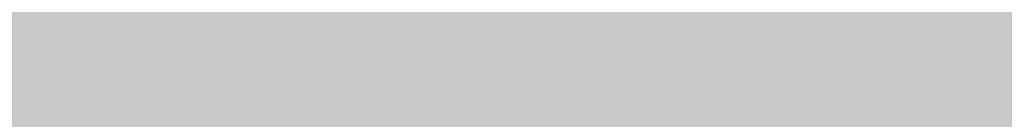
# Model space of a CAD drawing. Units: millimetres. Extents: x 0 to 2267, y 0 to 1823.
# Tile 101 of 256: x 1600.369 to 1605.705, y 1227.736 to 1228.277. Entities that reach past the tile are written whole.
import ezdxf

# ---------------------------------------------------------------- set-up
doc = ezdxf.new("R2010")
doc.units = ezdxf.units.MM
doc.header["$MEASUREMENT"] = 0
doc.layers.add('M-DIMS', color=2, linetype='Continuous', lineweight=25)
doc.layers.add('M-HATC', color=252, linetype='Continuous', lineweight=18)
doc.styles.get("Standard").update_dxf_attribs({"font": 'arial.ttf'})
doc.dimstyles.get("Standard").update_dxf_attribs({"dimtxt": 7, "dimasz": 4, "dimexe": 0.18, "dimexo": 0.0625, "dimgap": 0.09, "dimtad": 0, "dimdec": 0, "dimzin": 0, "dimdsep": 46, "dimtxsty": 'Standard', "dimcen": 0.09, "dimadec": 0, "dimazin": 0, "dimtfac": 1, "dimtdec": 0, "dimtofl": 0, "dimtmove": 0, "dimatfit": 3, "dimfxl": 1, "dimtolj": 1, "dimtzin": 0, "dimarcsym": 0})

# ---------------------------------------------------------------- blocks, each defined once
blk = doc.blocks.new('*D19')
at = {"layer": 'Defpoints', "color": 0, "transparency": 16777216}
for p in [(1605.3399, 1483.3044), (1445.5291, 1333.8851)]:
    blk.add_point(p, dxfattribs=at)
at = {"layer": 'M-DIMS', "color": 0, "lineweight": -2, "transparency": 16777216}
for p, q in [((1605.3399, 1483.2144), (1605.3399, 1483.3944)), ((1605.2499, 1483.3044), (1605.4299, 1483.3044)), ((1366.3244, 1259.8306), (1442.6072, 1331.1532))]:
    blk.add_line(p, q, dxfattribs=at)
at = {"layer": 'M-DIMS', "color": 0, "transparency": 16777216}
blk.add_solid([(1442.1519, 1331.6402), (1443.0625, 1330.6663), (1445.5291, 1333.8851)], dxfattribs=at)
at = {"layer": 'M-DIMS', "color": 0, "transparency": 16777216, "insert": (1349.6425, 1244.2335), "char_height": 7, "attachment_point": 5, "rotation": 43.0753}
blk.add_mtext('\\A1;2X R218.8', dxfattribs=at)

msp = doc.modelspace()

# ---------------------------------------------------------------- hatches: boundary and pattern name
at = {"layer": 'M-HATC'}
h = msp.add_hatch(color=256, dxfattribs=at)
h.dxf.hatch_style = 1
h.paths.add_polyline_path([(2055.771, 1603.062), (1381.0868, 1603.062), (1381.0868, 1598.062), (2055.771, 1598.062)])
h.paths.add_polyline_path([(2055.771, 1598.062), (1381.0868, 1598.062), (1381.0868, 1593.062), (2055.771, 1593.062)])
h.paths.add_polyline_path([(2051.3074, 1536.7609), (1385.5504, 1536.7609), (1385.5504, 1526.7609), (1387.5504, 1526.7609), (1388.5366, 1525.0528), (1385.3319, 1521.2335), (1385.3319, 1521.2226), (2050.2542, 1522.7491), (2048.3212, 1525.0528), (2049.3074, 1526.7609), (2051.3074, 1526.7609)])
edge = h.paths.add_edge_path()
edge.add_arc((1847.5345, 1379.1492), 135, 222.603061, 222.890851, ccw=False)
edge.add_line((1748.1663, 1287.7656), (1683.0921, 1287.7656))
edge.add_arc((1583.7239, 1379.1492), 135, 317.109149, 317.396939, ccw=False)
edge.add_arc((1678.9686, 1290.6707), 5, 222.8909, 317.1091, ccw=False)
edge.add_arc((1774.2133, 1379.1492), 135, 222.603061, 222.890851, ccw=False)
edge.add_line((1674.8451, 1287.7656), (1609.7709, 1287.7656))
edge.add_arc((1510.4027, 1379.1492), 135, 317.109149, 317.396939, ccw=False)
edge.add_arc((1605.6474, 1290.6707), 5, 222.8909, 317.1091, ccw=False)
edge.add_arc((1700.8921, 1379.1492), 135, 222.603061, 222.890851, ccw=False)
edge.add_line((1601.5239, 1287.7656), (1536.4497, 1287.7656))
edge.add_arc((1437.0815, 1379.1492), 135, 317.109149, 317.396939, ccw=False)
edge.add_arc((1532.3262, 1290.6707), 5, 222.8909, 317.1091, ccw=False)
edge.add_arc((1627.5709, 1379.1492), 135, 222.603061, 222.890851, ccw=False)
edge.add_line((1528.2027, 1287.7656), (1505.9289, 1287.7656))
edge.add_spline(control_points=[(1505.9289, 1287.7656), (1504.2622, 1287.7656), (1504.2622, 1282.7656), (1505.9289, 1282.7656)], knot_values=[0, 0, 0, 0, 5, 5, 5, 5], degree=3, periodic=0)
edge.add_line((1505.9289, 1282.7656), (1930.9289, 1282.7656))
edge.add_spline(control_points=[(1930.9289, 1282.7656), (1932.5956, 1282.7656), (1932.5956, 1287.7656), (1930.9289, 1287.7656)], knot_values=[0, 0, 0, 0, 5, 5, 5, 5], degree=3, periodic=0)
edge.add_line((1930.9289, 1287.7656), (1903.0557, 1287.7656))
edge.add_arc((1803.6875, 1379.1492), 135, 317.109149, 317.396939, ccw=False)
edge.add_arc((1898.9322, 1290.6707), 5, 222.8909, 317.1091, ccw=False)
edge.add_arc((1994.1769, 1379.1492), 135, 222.603061, 222.890851, ccw=False)
edge.add_line((1894.8087, 1287.7656), (1829.7345, 1287.7656))
edge.add_arc((1730.3663, 1379.1492), 135, 317.109149, 317.396939, ccw=False)
edge.add_arc((1825.611, 1290.6707), 5, 222.8909, 317.1091, ccw=False)
edge.add_arc((1920.8557, 1379.1492), 135, 222.603061, 222.890851, ccw=False)
edge.add_line((1821.4875, 1287.7656), (1756.4133, 1287.7656))
edge.add_arc((1657.0451, 1379.1492), 135, 317.109149, 317.396939, ccw=False)
edge.add_arc((1752.2898, 1290.6707), 5, 222.8909, 317.1091, ccw=False)
edge = h.paths.add_edge_path()
edge.add_spline(control_points=[(1843.4289, 1227.2475), (1845.0956, 1227.2475), (1845.0956, 1232.2475), (1843.4289, 1232.2475)], knot_values=[0, 0, 0, 0, 5, 5, 5, 5], degree=3, periodic=0)
edge.add_line((1843.4289, 1232.2475), (1593.4289, 1232.2475))
edge.add_spline(control_points=[(1593.4289, 1232.2475), (1591.7622, 1232.2475), (1591.7622, 1227.2475), (1593.4289, 1227.2475)], knot_values=[0, 0, 0, 0, 5, 5, 5, 5], degree=3, periodic=0)
edge.add_line((1593.4289, 1227.2475), (1843.4289, 1227.2475))
h.paths.add_polyline_path([(1905.9289, 1127.4171), (1530.9289, 1127.4171, 0.414214), (1520.9289, 1117.4171), (1530.9289, 1117.4171), (1915.9289, 1117.4171, 0.414214)])
edge = h.paths.add_edge_path()
edge.add_arc((1397.0858, 1498.4078), 12.7299, 90.78215, 190.87871, ccw=False)
edge.add_line((1396.912, 1511.1365), (1428.0097, 1511.3488))
edge.add_line((1428.0097, 1511.3488), (1433.0097, 1511.3488))
edge.add_line((1433.0097, 1511.3488), (1434.439, 1511.3488))
edge.add_arc((1419.474, 1498.0804), 20, 41.561, 74.08211)
edge.add_line((1424.9592, 1517.3135), (1399.9351, 1517.2561))
edge.add_spline(control_points=[(1399.9307, 1517.2561), (1399.884, 1517.2131), (1399.8328, 1517.1689), (1399.7774, 1517.1236)], knot_values=[11.567499, 11.567499, 11.567499, 11.567499, 11.814249, 11.814249, 11.814249, 11.814249], degree=3, periodic=0)
edge.add_spline(control_points=[(1399.6328, 1517.0099), (1399.5831, 1516.9721), (1399.5307, 1516.9338), (1399.4759, 1516.8947)], knot_values=[11.167718, 11.167718, 11.167718, 11.167718, 11.365188, 11.365188, 11.365188, 11.365188], degree=3, periodic=0)
edge.add_spline(control_points=[(1399.3398, 1516.8001), (1399.1514, 1516.6719), (1398.9384, 1516.5377), (1398.704, 1516.3994)], knot_values=[10.376405, 10.376405, 10.376405, 10.376405, 11.00994, 11.00994, 11.00994, 11.00994], degree=3, periodic=0)
edge.add_spline(control_points=[(1398.6572, 1516.3719), (1398.5789, 1516.326), (1398.4983, 1516.2797), (1398.4155, 1516.2331)], knot_values=[10.125175, 10.125175, 10.125175, 10.125175, 10.334406, 10.334406, 10.334406, 10.334406], degree=3, periodic=0)
edge.add_spline(control_points=[(1398.2642, 1516.1487), (1398.196, 1516.1111), (1398.1263, 1516.0732), (1398.0555, 1516.0351)], knot_values=[9.832246, 9.832246, 9.832246, 9.832246, 9.999658, 9.999658, 9.999658, 9.999658], degree=3, periodic=0)
edge.add_spline(control_points=[(1397.9987, 1516.0048), (1397.7312, 1515.8621), (1397.446, 1515.7171), (1397.1466, 1515.5714)], knot_values=[9.161808, 9.161808, 9.161808, 9.161808, 9.787769, 9.787769, 9.787769, 9.787769], degree=3, periodic=0)
edge.add_spline(control_points=[(1397.1466, 1515.5714), (1396.8418, 1515.423), (1396.5222, 1515.274), (1396.1914, 1515.1262)], knot_values=[8.524455, 8.524455, 8.524455, 8.524455, 9.161808, 9.161808, 9.161808, 9.161808], degree=3, periodic=0)
edge.add_spline(control_points=[(1396.0777, 1515.0756), (1395.9854, 1515.0348), (1395.8922, 1514.994), (1395.7983, 1514.9534)], knot_values=[8.275193, 8.275193, 8.275193, 8.275193, 8.451726, 8.451726, 8.451726, 8.451726], degree=3, periodic=0)
edge.add_spline(control_points=[(1395.6018, 1514.8691), (1395.4997, 1514.8257), (1395.3968, 1514.7824), (1395.2932, 1514.7394)], knot_values=[7.962917, 7.962917, 7.962917, 7.962917, 8.152764, 8.152764, 8.152764, 8.152764], degree=3, periodic=0)
edge.add_spline(control_points=[(1395.2116, 1514.7057), (1394.8278, 1514.5475), (1394.4345, 1514.3929), (1394.0364, 1514.2442)], knot_values=[7.21254, 7.21254, 7.21254, 7.21254, 7.913148, 7.913148, 7.913148, 7.913148], degree=3, periodic=0)
edge.add_spline(control_points=[(1394.0364, 1514.2442), (1393.7076, 1514.1214), (1393.3754, 1514.0027), (1393.0427, 1513.8895)], knot_values=[6.633733, 6.633733, 6.633733, 6.633733, 7.21254, 7.21254, 7.21254, 7.21254], degree=3, periodic=0)
edge.add_spline(control_points=[(1392.8214, 1513.815), (1392.7198, 1513.7812), (1392.6181, 1513.7479), (1392.5166, 1513.7152)], knot_values=[6.328796, 6.328796, 6.328796, 6.328796, 6.505493, 6.505493, 6.505493, 6.505493], degree=3, periodic=0)
edge.add_spline(control_points=[(1392.5166, 1513.7152), (1392.3187, 1513.6515), (1392.1212, 1513.59), (1391.9244, 1513.531)], knot_values=[5.984605, 5.984605, 5.984605, 5.984605, 6.328796, 6.328796, 6.328796, 6.328796], degree=3, periodic=0)
edge.add_spline(control_points=[(1391.7915, 1513.4915), (1391.3122, 1513.3501), (1390.8384, 1513.2239), (1390.3784, 1513.1171)], knot_values=[5.066697, 5.066697, 5.066697, 5.066697, 5.907055, 5.907055, 5.907055, 5.907055], degree=3, periodic=0)
edge.add_spline(control_points=[(1390.3784, 1513.1171), (1390.1797, 1513.071), (1389.9836, 1513.0284), (1389.7907, 1512.9899)], knot_values=[4.70367, 4.70367, 4.70367, 4.70367, 5.066695, 5.066695, 5.066695, 5.066695], degree=3, periodic=0)
edge.add_spline(control_points=[(1389.422, 1512.9204), (1389.2459, 1512.8892), (1389.0729, 1512.8617), (1388.9036, 1512.8381)], knot_values=[4.130571, 4.130571, 4.130571, 4.130571, 4.469816, 4.469816, 4.469816, 4.469816], degree=3, periodic=0)
edge.add_spline(control_points=[(1388.9036, 1512.8381), (1388.591, 1512.7946), (1388.2911, 1512.7644), (1388.0071, 1512.7494)], knot_values=[3.504031, 3.504031, 3.504031, 3.504031, 4.130571, 4.130571, 4.130571, 4.130571], degree=3, periodic=0)
edge.add_spline(control_points=[(1387.9356, 1512.7459), (1387.8538, 1512.7423), (1387.7733, 1512.74), (1387.6944, 1512.739)], knot_values=[3.268866, 3.268866, 3.268866, 3.268866, 3.451164, 3.451164, 3.451164, 3.451164], degree=3, periodic=0)
edge.add_spline(control_points=[(1387.3351, 1512.7443), (1387.2076, 1512.7499), (1387.0847, 1512.7597), (1386.967, 1512.7739)], knot_values=[2.670686, 2.670686, 2.670686, 2.670686, 2.984, 2.984, 2.984, 2.984], degree=3, periodic=0)
edge.add_spline(control_points=[(1386.8327, 1512.7922), (1386.8209, 1512.7941), (1386.8092, 1512.7959), (1386.7975, 1512.7979)], knot_values=[2.516981, 2.516981, 2.516981, 2.516981, 2.549528, 2.549528, 2.549528, 2.549528], degree=3, periodic=0)
edge.add_spline(control_points=[(1386.4526, 1512.8735), (1386.4257, 1512.881), (1386.3993, 1512.889), (1386.3733, 1512.8972)], knot_values=[2.095869, 2.095869, 2.095869, 2.095869, 2.17941, 2.17941, 2.17941, 2.17941], degree=3, periodic=0)
edge.add_spline(control_points=[(1386.0691, 1513.0189), (1386.0634, 1513.0217), (1386.0577, 1513.0246), (1386.052, 1513.0275)], knot_values=[1.72453, 1.72453, 1.72453, 1.72453, 1.745933, 1.745933, 1.745933, 1.745933], degree=3, periodic=0)
edge.add_arc((1399.474, 1498.0804), 20, 131.82432, 180)
edge.add_arc((1630.3336, 1505.5484), 250.9708, 181.705176, 236.427975)
edge.add_arc((1605.3399, 1483.3044), 218.7822, 238.660829, 243.34961)
edge.add_arc((1647.0911, 1510.3592), 262.8986, 183.129836, 237.853442, ccw=False)
h.paths.add_polyline_path([(1406.5369, 1391.9644, 0.149382), (1491.5506, 1296.4418, -0.129517)], flags=17)
edge = h.paths.add_edge_path()
edge.add_arc((2037.3838, 1498.0804), 20, 0, 48.26587)
edge.add_spline(control_points=[(2050.6973, 1513.0052), (2050.6512, 1512.9847), (2050.6034, 1512.9655), (2050.5539, 1512.9477)], knot_values=[1.835652, 1.835652, 1.835652, 1.835652, 2.000781, 2.000781, 2.000781, 2.000781], degree=3, periodic=0)
edge.add_spline(control_points=[(2050.4616, 1512.9166), (2050.479, 1512.9221), (2050.4963, 1512.9277), (2050.5133, 1512.9335)], knot_values=[2.045477, 2.045477, 2.045477, 2.045477, 2.101389, 2.101389, 2.101389, 2.101389], degree=3, periodic=0)
edge.add_spline(control_points=[(2050.129, 1512.8342), (2050.1984, 1512.8473), (2050.2657, 1512.8623), (2050.3308, 1512.8792)], knot_values=[2.237629, 2.237629, 2.237629, 2.237629, 2.435841, 2.435841, 2.435841, 2.435841], degree=3, periodic=0)
edge.add_spline(control_points=[(2050.0946, 1512.8278), (2050.1061, 1512.8299), (2050.1176, 1512.832), (2050.129, 1512.8342)], knot_values=[2.435841, 2.435841, 2.435841, 2.435841, 2.468321, 2.468321, 2.468321, 2.468321], degree=3, periodic=0)
edge.add_spline(control_points=[(2049.7843, 1512.7851), (2049.8552, 1512.7922), (2049.9243, 1512.8008), (2049.9917, 1512.8109)], knot_values=[2.563852, 2.563852, 2.563852, 2.563852, 2.748541, 2.748541, 2.748541, 2.748541], degree=3, periodic=0)
edge.add_spline(control_points=[(2049.4052, 1512.7617), (2049.5364, 1512.7653), (2049.6629, 1512.773), (2049.7843, 1512.7851)], knot_values=[2.748541, 2.748541, 2.748541, 2.748541, 3.064882, 3.064882, 3.064882, 3.064882], degree=3, periodic=0)
edge.add_spline(control_points=[(2049.1698, 1512.7597), (2049.2336, 1512.7591), (2049.2965, 1512.7594), (2049.3584, 1512.7606)], knot_values=[3.102309, 3.102309, 3.102309, 3.102309, 3.2503, 3.2503, 3.2503, 3.2503], degree=3, periodic=0)
edge.add_spline(control_points=[(2048.8573, 1512.7691), (2048.9638, 1512.7638), (2049.068, 1512.7606), (2049.1698, 1512.7597)], knot_values=[3.2503, 3.2503, 3.2503, 3.2503, 3.486069, 3.486069, 3.486069, 3.486069], degree=3, periodic=0)
edge.add_spline(control_points=[(2048.6924, 1512.7789), (2048.3729, 1512.8009), (2048.0345, 1512.8411), (2047.6817, 1512.897)], knot_values=[3.606429, 3.606429, 3.606429, 3.606429, 4.2989, 4.2989, 4.2989, 4.2989], degree=3, periodic=0)
edge.add_spline(control_points=[(2047.6817, 1512.897), (2047.5458, 1512.9185), (2047.4077, 1512.9424), (2047.2678, 1512.9685)], knot_values=[4.2989, 4.2989, 4.2989, 4.2989, 4.565769, 4.565769, 4.565769, 4.565769], degree=3, periodic=0)
edge.add_spline(control_points=[(2047.2678, 1512.9685), (2047.1449, 1512.9914), (2047.0207, 1513.016), (2046.8951, 1513.0422)], knot_values=[4.565769, 4.565769, 4.565769, 4.565769, 4.799971, 4.799971, 4.799971, 4.799971], degree=3, periodic=0)
edge.add_spline(control_points=[(2046.8951, 1513.0422), (2046.5286, 1513.1188), (2046.1513, 1513.209), (2045.7676, 1513.3107)], knot_values=[4.799971, 4.799971, 4.799971, 4.799971, 5.483718, 5.483718, 5.483718, 5.483718], degree=3, periodic=0)
edge.add_spline(control_points=[(2045.7676, 1513.3107), (2045.3724, 1513.4154), (2044.9704, 1513.5322), (2044.5662, 1513.6588)], knot_values=[5.483718, 5.483718, 5.483718, 5.483718, 6.187866, 6.187866, 6.187866, 6.187866], degree=3, periodic=0)
edge.add_spline(control_points=[(2044.5662, 1513.6588), (2044.4149, 1513.7061), (2044.2633, 1513.7549), (2044.1116, 1513.8048)], knot_values=[6.187866, 6.187866, 6.187866, 6.187866, 6.451551, 6.451551, 6.451551, 6.451551], degree=3, periodic=0)
edge.add_spline(control_points=[(2044.1116, 1513.8048), (2043.9967, 1513.8427), (2043.8817, 1513.8813), (2043.7668, 1513.9205)], knot_values=[6.451551, 6.451551, 6.451551, 6.451551, 6.651434, 6.651434, 6.651434, 6.651434], degree=3, periodic=0)
edge.add_spline(control_points=[(2043.7668, 1513.9205), (2043.3716, 1514.0554), (2042.9774, 1514.1979), (2042.5886, 1514.3458)], knot_values=[6.651434, 6.651434, 6.651434, 6.651434, 7.338879, 7.338879, 7.338879, 7.338879], degree=3, periodic=0)
edge.add_spline(control_points=[(2042.5886, 1514.3458), (2042.1643, 1514.5071), (2041.7465, 1514.6749), (2041.3409, 1514.846)], knot_values=[7.338879, 7.338879, 7.338879, 7.338879, 8.089209, 8.089209, 8.089209, 8.089209], degree=3, periodic=0)
edge.add_spline(control_points=[(2041.3409, 1514.846), (2041.1028, 1514.9465), (2040.869, 1515.0481), (2040.6405, 1515.1502)], knot_values=[8.089209, 8.089209, 8.089209, 8.089209, 8.529587, 8.529587, 8.529587, 8.529587], degree=3, periodic=0)
edge.add_spline(control_points=[(2040.51, 1515.2089), (2040.0824, 1515.4022), (2039.6747, 1515.5971), (2039.295, 1515.7894)], knot_values=[8.613818, 8.613818, 8.613818, 8.613818, 9.44571, 9.44571, 9.44571, 9.44571], degree=3, periodic=0)
edge.add_spline(control_points=[(2039.295, 1515.7894), (2039.0618, 1515.9075), (2038.8391, 1516.0246), (2038.6288, 1516.1398)], knot_values=[9.44571, 9.44571, 9.44571, 9.44571, 9.956404, 9.956404, 9.956404, 9.956404], degree=3, periodic=0)
edge.add_spline(control_points=[(2038.6288, 1516.1398), (2038.5187, 1516.2001), (2038.4121, 1516.2598), (2038.309, 1516.3189)], knot_values=[9.956404, 9.956404, 9.956404, 9.956404, 10.223542, 10.223542, 10.223542, 10.223542], degree=3, periodic=0)
edge.add_spline(control_points=[(2038.309, 1516.3189), (2038.2138, 1516.3735), (2038.1216, 1516.4276), (2038.0328, 1516.481)], knot_values=[10.223542, 10.223542, 10.223542, 10.223542, 10.47051, 10.47051, 10.47051, 10.47051], degree=3, periodic=0)
edge.add_spline(control_points=[(2038.0328, 1516.481), (2037.7855, 1516.6296), (2037.5639, 1516.773), (2037.3722, 1516.909)], knot_values=[10.47051, 10.47051, 10.47051, 10.47051, 11.15767, 11.15767, 11.15767, 11.15767], degree=3, periodic=0)
edge.add_spline(control_points=[(2037.3722, 1516.909), (2037.2789, 1516.9752), (2037.1927, 1517.0396), (2037.1142, 1517.102)], knot_values=[11.15767, 11.15767, 11.15767, 11.15767, 11.49227, 11.49227, 11.49227, 11.49227], degree=3, periodic=0)
edge.add_spline(control_points=[(2036.8564, 1517.3259), (2036.9148, 1517.2692), (2036.9814, 1517.2103), (2037.0557, 1517.1492)], knot_values=[11.577341, 11.577341, 11.577341, 11.577341, 11.91035, 11.91035, 11.91035, 11.91035], degree=3, periodic=0)
edge.add_spline(control_points=[(2036.8074, 1517.3748), (2036.823, 1517.3587), (2036.8393, 1517.3424), (2036.8564, 1517.3259)], knot_values=[11.91035, 11.91035, 11.91035, 11.91035, 12.007402, 12.007402, 12.007402, 12.007402], degree=3, periodic=0)
edge.add_spline(control_points=[(2036.7017, 1517.494), (2036.7104, 1517.483), (2036.7196, 1517.4719), (2036.7291, 1517.4606)], knot_values=[12.184155, 12.184155, 12.184155, 12.184155, 12.255409, 12.255409, 12.255409, 12.255409], degree=3, periodic=0)
edge.add_spline(control_points=[(2036.6159, 1517.6205), (2036.62, 1517.613), (2036.6243, 1517.6055), (2036.6289, 1517.5979)], knot_values=[12.487913, 12.487913, 12.487913, 12.487913, 12.541035, 12.541035, 12.541035, 12.541035], degree=3, periodic=0)
edge.add_spline(control_points=[(2036.5635, 1517.786), (2036.5637, 1517.7794), (2036.5642, 1517.7726), (2036.565, 1517.7658)], knot_values=[12.911761, 12.911761, 12.911761, 12.911761, 12.968286, 12.968286, 12.968286, 12.968286], degree=3, periodic=0)
edge.add_spline(control_points=[(2036.6166, 1517.9304), (2036.6125, 1517.9259), (2036.6086, 1517.9212), (2036.6049, 1517.9165)], knot_values=[13.382527, 13.382527, 13.382527, 13.382527, 13.433791, 13.433791, 13.433791, 13.433791], degree=3, periodic=0)
edge.add_spline(control_points=[(2036.749, 1518.017), (2036.7361, 1518.0116), (2036.7239, 1518.006), (2036.7124, 1518.0002)], knot_values=[13.726299, 13.726299, 13.726299, 13.726299, 13.809928, 13.809928, 13.809928, 13.809928], degree=3, periodic=0)
edge.add_spline(control_points=[(2036.8604, 1518.0528), (2036.8386, 1518.0474), (2036.8181, 1518.0416), (2036.7988, 1518.0353)], knot_values=[13.910887, 13.910887, 13.910887, 13.910887, 14.02153, 14.02153, 14.02153, 14.02153], degree=3, periodic=0)
edge.add_line((2036.9639, 1518.0804), (2032.3838, 1518.0804))
edge.add_line((2032.3838, 1518.0804), (2027.3838, 1518.0804))
edge.add_line((2027.3838, 1518.0804), (2022.3838, 1518.0804))
edge.add_line((2022.3838, 1518.0804), (2017.3838, 1518.0804))
edge.add_arc((2017.3838, 1498.0804), 20, 90, 138.439)
edge.add_line((2002.4188, 1511.3488), (2003.8481, 1511.3488))
edge.add_line((2003.8481, 1511.3488), (2008.8481, 1511.3488))
edge.add_line((2008.8481, 1511.3488), (2039.772, 1511.1377))
edge.add_arc((2039.772, 1498.4078), 12.7299, -10.87871, 90, ccw=False)
edge.add_arc((1789.7668, 1510.3592), 262.8986, 302.146558, 356.870164, ccw=False)
edge.add_arc((1831.5179, 1483.3044), 218.7822, 296.65039, 301.339171)
edge.add_arc((1806.5242, 1505.5484), 250.9708, 303.572025, 358.294824)
h.paths.add_polyline_path([(2030.321, 1391.9644, -0.129517), (1945.3072, 1296.4418, 0.149382)], flags=17)
edge = h.paths.add_edge_path()
edge.add_spline(control_points=[(2037.2464, 1518.0821), (2037.2898, 1518.081), (2037.3355, 1518.0804), (2037.3838, 1518.0804)], knot_values=[0.000012, 0.000012, 0.000012, 0.000012, 0.144754, 0.144754, 0.144754, 0.144754], degree=3, periodic=0)
edge.add_line((2037.3357, 1518.0804), (2037.0096, 1518.0804))
edge.add_spline(control_points=[(2037.0096, 1518.0804), (2036.9822, 1518.0768), (2036.956, 1518.0727), (2036.9312, 1518.0681)], knot_values=[14.13465, 14.13465, 14.13465, 14.13465, 14.247197, 14.247197, 14.247197, 14.247197], degree=3, periodic=0)
edge.add_spline(control_points=[(2036.9312, 1518.0681), (2036.9276, 1518.0674), (2036.9241, 1518.0667), (2036.9205, 1518.0661)], knot_values=[14.118315, 14.118315, 14.118315, 14.118315, 14.13465, 14.13465, 14.13465, 14.13465], degree=3, periodic=0)
edge.add_spline(control_points=[(2036.9205, 1518.0661), (2036.9118, 1518.0644), (2036.9032, 1518.0626), (2036.8948, 1518.0608)], knot_values=[14.078086, 14.078086, 14.078086, 14.078086, 14.118315, 14.118315, 14.118315, 14.118315], degree=3, periodic=0)
edge.add_spline(control_points=[(2036.8948, 1518.0608), (2036.883, 1518.0583), (2036.8716, 1518.0556), (2036.8604, 1518.0528)], knot_values=[14.02153, 14.02153, 14.02153, 14.02153, 14.078086, 14.078086, 14.078086, 14.078086], degree=3, periodic=0)
edge.add_spline(control_points=[(2036.8604, 1518.0528), (2036.8386, 1518.0474), (2036.8181, 1518.0416), (2036.7988, 1518.0353)], knot_values=[13.910887, 13.910887, 13.910887, 13.910887, 14.02153, 14.02153, 14.02153, 14.02153], degree=3, periodic=0)
edge.add_spline(control_points=[(2036.7988, 1518.0353), (2036.7981, 1518.035), (2036.7974, 1518.0348), (2036.7967, 1518.0346)], knot_values=[13.906906, 13.906906, 13.906906, 13.906906, 13.910887, 13.910887, 13.910887, 13.910887], degree=3, periodic=0)
edge.add_spline(control_points=[(2036.7967, 1518.0346), (2036.7882, 1518.0318), (2036.7799, 1518.0289), (2036.7719, 1518.0259)], knot_values=[13.857826, 13.857826, 13.857826, 13.857826, 13.906906, 13.906906, 13.906906, 13.906906], degree=3, periodic=0)
edge.add_spline(control_points=[(2036.7719, 1518.0259), (2036.764, 1518.023), (2036.7564, 1518.02), (2036.749, 1518.017)], knot_values=[13.809928, 13.809928, 13.809928, 13.809928, 13.857826, 13.857826, 13.857826, 13.857826], degree=3, periodic=0)
edge.add_spline(control_points=[(2036.749, 1518.017), (2036.7361, 1518.0116), (2036.7239, 1518.006), (2036.7124, 1518.0002)], knot_values=[13.726299, 13.726299, 13.726299, 13.726299, 13.809928, 13.809928, 13.809928, 13.809928], degree=3, periodic=0)
edge.add_spline(control_points=[(2036.7124, 1518.0002), (2036.7121, 1518), (2036.7118, 1517.9999), (2036.7115, 1517.9997)], knot_values=[13.723993, 13.723993, 13.723993, 13.723993, 13.726299, 13.726299, 13.726299, 13.726299], degree=3, periodic=0)
edge.add_spline(control_points=[(2036.7115, 1517.9997), (2036.7063, 1517.9971), (2036.7013, 1517.9944), (2036.6965, 1517.9917)], knot_values=[13.686536, 13.686536, 13.686536, 13.686536, 13.723993, 13.723993, 13.723993, 13.723993], degree=3, periodic=0)
edge.add_spline(control_points=[(2036.6965, 1517.9917), (2036.6919, 1517.9891), (2036.6874, 1517.9865), (2036.6831, 1517.9839)], knot_values=[13.651251, 13.651251, 13.651251, 13.651251, 13.686536, 13.686536, 13.686536, 13.686536], degree=3, periodic=0)
edge.add_spline(control_points=[(2036.6831, 1517.9839), (2036.6764, 1517.9798), (2036.67, 1517.9757), (2036.6639, 1517.9714)], knot_values=[13.596804, 13.596804, 13.596804, 13.596804, 13.651251, 13.651251, 13.651251, 13.651251], degree=3, periodic=0)
edge.add_spline(control_points=[(2036.6639, 1517.9714), (2036.6636, 1517.9712), (2036.6633, 1517.9709), (2036.6629, 1517.9707)], knot_values=[13.593956, 13.593956, 13.593956, 13.593956, 13.596804, 13.596804, 13.596804, 13.596804], degree=3, periodic=0)
edge.add_spline(control_points=[(2036.6629, 1517.9707), (2036.6603, 1517.9689), (2036.6577, 1517.967), (2036.6552, 1517.9651)], knot_values=[13.570322, 13.570322, 13.570322, 13.570322, 13.593956, 13.593956, 13.593956, 13.593956], degree=3, periodic=0)
edge.add_spline(control_points=[(2036.6552, 1517.9651), (2036.6525, 1517.9631), (2036.6499, 1517.9611), (2036.6474, 1517.9591)], knot_values=[13.545477, 13.545477, 13.545477, 13.545477, 13.570322, 13.570322, 13.570322, 13.570322], degree=3, periodic=0)
edge.add_spline(control_points=[(2036.6474, 1517.9591), (2036.6472, 1517.9589), (2036.6471, 1517.9588), (2036.6469, 1517.9587)], knot_values=[13.543931, 13.543931, 13.543931, 13.543931, 13.545477, 13.545477, 13.545477, 13.545477], degree=3, periodic=0)
edge.add_spline(control_points=[(2036.6469, 1517.9587), (2036.6412, 1517.9541), (2036.6358, 1517.9494), (2036.6307, 1517.9447)], knot_values=[13.488237, 13.488237, 13.488237, 13.488237, 13.543931, 13.543931, 13.543931, 13.543931], degree=3, periodic=0)
edge.add_spline(control_points=[(2036.6307, 1517.9447), (2036.6282, 1517.9423), (2036.6257, 1517.9399), (2036.6233, 1517.9374)], knot_values=[13.460307, 13.460307, 13.460307, 13.460307, 13.488237, 13.488237, 13.488237, 13.488237], degree=3, periodic=0)
edge.add_spline(control_points=[(2036.6233, 1517.9374), (2036.6215, 1517.9356), (2036.6198, 1517.9338), (2036.6181, 1517.932)], knot_values=[13.439712, 13.439712, 13.439712, 13.439712, 13.460307, 13.460307, 13.460307, 13.460307], degree=3, periodic=0)
edge.add_spline(control_points=[(2036.6181, 1517.932), (2036.6176, 1517.9315), (2036.6171, 1517.9309), (2036.6166, 1517.9304)], knot_values=[13.433791, 13.433791, 13.433791, 13.433791, 13.439712, 13.439712, 13.439712, 13.439712], degree=3, periodic=0)
edge.add_spline(control_points=[(2036.6166, 1517.9304), (2036.6125, 1517.9259), (2036.6086, 1517.9212), (2036.6049, 1517.9165)], knot_values=[13.382527, 13.382527, 13.382527, 13.382527, 13.433791, 13.433791, 13.433791, 13.433791], degree=3, periodic=0)
edge.add_spline(control_points=[(2036.6049, 1517.9165), (2036.6026, 1517.9135), (2036.6004, 1517.9104), (2036.5982, 1517.9074)], knot_values=[13.350017, 13.350017, 13.350017, 13.350017, 13.382527, 13.382527, 13.382527, 13.382527], degree=3, periodic=0)
edge.add_spline(control_points=[(2036.5982, 1517.9074), (2036.5972, 1517.9059), (2036.5962, 1517.9043), (2036.5952, 1517.9028)], knot_values=[13.333922, 13.333922, 13.333922, 13.333922, 13.350017, 13.350017, 13.350017, 13.350017], degree=3, periodic=0)
edge.add_spline(control_points=[(2036.5952, 1517.9028), (2036.5945, 1517.9018), (2036.5939, 1517.9009), (2036.5933, 1517.8999)], knot_values=[13.323828, 13.323828, 13.323828, 13.323828, 13.333922, 13.333922, 13.333922, 13.333922], degree=3, periodic=0)
edge.add_spline(control_points=[(2036.5933, 1517.8999), (2036.5905, 1517.8955), (2036.5879, 1517.8909), (2036.5855, 1517.8864)], knot_values=[13.277545, 13.277545, 13.277545, 13.277545, 13.323828, 13.323828, 13.323828, 13.323828], degree=3, periodic=0)
edge.add_spline(control_points=[(2036.5855, 1517.8864), (2036.5836, 1517.8827), (2036.5817, 1517.8789), (2036.5801, 1517.8751)], knot_values=[13.240119, 13.240119, 13.240119, 13.240119, 13.277545, 13.277545, 13.277545, 13.277545], degree=3, periodic=0)
edge.add_spline(control_points=[(2036.5801, 1517.8751), (2036.5795, 1517.8739), (2036.579, 1517.8727), (2036.5785, 1517.8715)], knot_values=[13.228211, 13.228211, 13.228211, 13.228211, 13.240119, 13.240119, 13.240119, 13.240119], degree=3, periodic=0)
edge.add_spline(control_points=[(2036.5785, 1517.8715), (2036.578, 1517.8702), (2036.5774, 1517.869), (2036.5769, 1517.8677)], knot_values=[13.215717, 13.215717, 13.215717, 13.215717, 13.228211, 13.228211, 13.228211, 13.228211], degree=3, periodic=0)
edge.add_spline(control_points=[(2036.5769, 1517.8677), (2036.5755, 1517.864), (2036.5741, 1517.8603), (2036.5729, 1517.8565)], knot_values=[13.179847, 13.179847, 13.179847, 13.179847, 13.215717, 13.215717, 13.215717, 13.215717], degree=3, periodic=0)
edge.add_spline(control_points=[(2036.5729, 1517.8565), (2036.5713, 1517.8515), (2036.5699, 1517.8464), (2036.5687, 1517.8413)], knot_values=[13.132017, 13.132017, 13.132017, 13.132017, 13.179847, 13.179847, 13.179847, 13.179847], degree=3, periodic=0)
edge.add_spline(control_points=[(2036.5687, 1517.8413), (2036.5684, 1517.8402), (2036.5682, 1517.8392), (2036.568, 1517.8382)], knot_values=[13.122482, 13.122482, 13.122482, 13.122482, 13.132017, 13.132017, 13.132017, 13.132017], degree=3, periodic=0)
edge.add_spline(control_points=[(2036.568, 1517.8382), (2036.5676, 1517.8363), (2036.5672, 1517.8345), (2036.5669, 1517.8327)], knot_values=[13.105592, 13.105592, 13.105592, 13.105592, 13.122482, 13.122482, 13.122482, 13.122482], degree=3, periodic=0)
edge.add_spline(control_points=[(2036.5669, 1517.8327), (2036.5662, 1517.8292), (2036.5657, 1517.8257), (2036.5652, 1517.8222)], knot_values=[13.074063, 13.074063, 13.074063, 13.074063, 13.105592, 13.105592, 13.105592, 13.105592], degree=3, periodic=0)
edge.add_spline(control_points=[(2036.5652, 1517.8222), (2036.5652, 1517.8222), (2036.5652, 1517.8222), (2036.5652, 1517.8222)], knot_values=[13.074043, 13.074043, 13.074043, 13.074043, 13.074063, 13.074063, 13.074063, 13.074063], degree=3, periodic=0)
edge.add_spline(control_points=[(2036.5652, 1517.8222), (2036.5644, 1517.8164), (2036.5639, 1517.8106), (2036.5636, 1517.8046)], knot_values=[13.021884, 13.021884, 13.021884, 13.021884, 13.074043, 13.074043, 13.074043, 13.074043], degree=3, periodic=0)
edge.add_spline(control_points=[(2036.5636, 1517.8046), (2036.5636, 1517.804), (2036.5636, 1517.8034), (2036.5635, 1517.8028)], knot_values=[13.01674, 13.01674, 13.01674, 13.01674, 13.021884, 13.021884, 13.021884, 13.021884], degree=3, periodic=0)
edge.add_spline(control_points=[(2036.5635, 1517.8028), (2036.5634, 1517.8005), (2036.5634, 1517.7982), (2036.5634, 1517.7958)], knot_values=[12.996438, 12.996438, 12.996438, 12.996438, 13.01674, 13.01674, 13.01674, 13.01674], degree=3, periodic=0)
edge.add_spline(control_points=[(2036.5634, 1517.7958), (2036.5633, 1517.7926), (2036.5634, 1517.7893), (2036.5635, 1517.786)], knot_values=[12.968286, 12.968286, 12.968286, 12.968286, 12.996438, 12.996438, 12.996438, 12.996438], degree=3, periodic=0)
edge.add_spline(control_points=[(2036.5635, 1517.786), (2036.5637, 1517.7794), (2036.5642, 1517.7726), (2036.565, 1517.7658)], knot_values=[12.911761, 12.911761, 12.911761, 12.911761, 12.968286, 12.968286, 12.968286, 12.968286], degree=3, periodic=0)
edge.add_spline(control_points=[(2036.565, 1517.7658), (2036.565, 1517.7657), (2036.565, 1517.7656), (2036.565, 1517.7656)], knot_values=[12.911017, 12.911017, 12.911017, 12.911017, 12.911761, 12.911761, 12.911761, 12.911761], degree=3, periodic=0)
edge.add_spline(control_points=[(2036.565, 1517.7656), (2036.5654, 1517.7625), (2036.5658, 1517.7593), (2036.5663, 1517.7562)], knot_values=[12.88528, 12.88528, 12.88528, 12.88528, 12.911017, 12.911017, 12.911017, 12.911017], degree=3, periodic=0)
edge.add_spline(control_points=[(2036.5663, 1517.7562), (2036.5667, 1517.7534), (2036.5672, 1517.7506), (2036.5677, 1517.7478)], knot_values=[12.862519, 12.862519, 12.862519, 12.862519, 12.88528, 12.88528, 12.88528, 12.88528], degree=3, periodic=0)
edge.add_spline(control_points=[(2036.5677, 1517.7478), (2036.5678, 1517.7474), (2036.5679, 1517.7469), (2036.568, 1517.7465)], knot_values=[12.858885, 12.858885, 12.858885, 12.858885, 12.862519, 12.862519, 12.862519, 12.862519], degree=3, periodic=0)
edge.add_spline(control_points=[(2036.568, 1517.7465), (2036.5692, 1517.7399), (2036.5707, 1517.7332), (2036.5724, 1517.7264)], knot_values=[12.8053, 12.8053, 12.8053, 12.8053, 12.858885, 12.858885, 12.858885, 12.858885], degree=3, periodic=0)
edge.add_spline(control_points=[(2036.5724, 1517.7264), (2036.5734, 1517.7226), (2036.5745, 1517.7187), (2036.5756, 1517.7149)], knot_values=[12.775176, 12.775176, 12.775176, 12.775176, 12.8053, 12.8053, 12.8053, 12.8053], degree=3, periodic=0)
edge.add_spline(control_points=[(2036.5756, 1517.7149), (2036.5763, 1517.7125), (2036.577, 1517.7102), (2036.5778, 1517.7078)], knot_values=[12.756759, 12.756759, 12.756759, 12.756759, 12.775176, 12.775176, 12.775176, 12.775176], degree=3, periodic=0)
edge.add_spline(control_points=[(2036.5778, 1517.7078), (2036.5781, 1517.7067), (2036.5784, 1517.7057), (2036.5787, 1517.7047)], knot_values=[12.748742, 12.748742, 12.748742, 12.748742, 12.756759, 12.756759, 12.756759, 12.756759], degree=3, periodic=0)
edge.add_spline(control_points=[(2036.5787, 1517.7047), (2036.5808, 1517.6983), (2036.5831, 1517.6919), (2036.5856, 1517.6854)], knot_values=[12.69959, 12.69959, 12.69959, 12.69959, 12.748742, 12.748742, 12.748742, 12.748742], degree=3, periodic=0)
edge.add_spline(control_points=[(2036.5856, 1517.6854), (2036.5876, 1517.68), (2036.5898, 1517.6746), (2036.5921, 1517.6692)], knot_values=[12.659038, 12.659038, 12.659038, 12.659038, 12.69959, 12.69959, 12.69959, 12.69959], degree=3, periodic=0)
edge.add_spline(control_points=[(2036.5921, 1517.6692), (2036.594, 1517.6648), (2036.5959, 1517.6605), (2036.5979, 1517.6561)], knot_values=[12.626806, 12.626806, 12.626806, 12.626806, 12.659038, 12.659038, 12.659038, 12.659038], degree=3, periodic=0)
edge.add_spline(control_points=[(2036.5979, 1517.6561), (2036.5984, 1517.6551), (2036.5989, 1517.6541), (2036.5993, 1517.6531)], knot_values=[12.619394, 12.619394, 12.619394, 12.619394, 12.626806, 12.626806, 12.626806, 12.626806], degree=3, periodic=0)
edge.add_spline(control_points=[(2036.5993, 1517.6531), (2036.6043, 1517.6424), (2036.6099, 1517.6315), (2036.6159, 1517.6205)], knot_values=[12.541039, 12.541039, 12.541039, 12.541039, 12.619394, 12.619394, 12.619394, 12.619394], degree=3, periodic=0)
edge.add_spline(control_points=[(2036.6159, 1517.6205), (2036.6159, 1517.6205), (2036.6159, 1517.6205), (2036.6159, 1517.6205)], knot_values=[12.541035, 12.541035, 12.541035, 12.541035, 12.541039, 12.541039, 12.541039, 12.541039], degree=3, periodic=0)
edge.add_spline(control_points=[(2036.6159, 1517.6205), (2036.62, 1517.613), (2036.6243, 1517.6055), (2036.6289, 1517.5979)], knot_values=[12.487913, 12.487913, 12.487913, 12.487913, 12.541035, 12.541035, 12.541035, 12.541035], degree=3, periodic=0)
edge.add_spline(control_points=[(2036.6289, 1517.5979), (2036.6326, 1517.5916), (2036.6365, 1517.5853), (2036.6406, 1517.5789)], knot_values=[12.443982, 12.443982, 12.443982, 12.443982, 12.487913, 12.487913, 12.487913, 12.487913], degree=3, periodic=0)
edge.add_spline(control_points=[(2036.6406, 1517.5789), (2036.6414, 1517.5776), (2036.6423, 1517.5763), (2036.6431, 1517.5749)], knot_values=[12.434996, 12.434996, 12.434996, 12.434996, 12.443982, 12.443982, 12.443982, 12.443982], degree=3, periodic=0)
edge.add_spline(control_points=[(2036.6431, 1517.5749), (2036.6531, 1517.5596), (2036.6639, 1517.5439), (2036.6756, 1517.528)], knot_values=[12.329647, 12.329647, 12.329647, 12.329647, 12.434996, 12.434996, 12.434996, 12.434996], degree=3, periodic=0)
edge.add_spline(control_points=[(2036.6756, 1517.528), (2036.6839, 1517.5168), (2036.6925, 1517.5055), (2036.7017, 1517.494)], knot_values=[12.255409, 12.255409, 12.255409, 12.255409, 12.329647, 12.329647, 12.329647, 12.329647], degree=3, periodic=0)
edge.add_spline(control_points=[(2036.7017, 1517.494), (2036.7104, 1517.483), (2036.7196, 1517.4719), (2036.7291, 1517.4606)], knot_values=[12.184155, 12.184155, 12.184155, 12.184155, 12.255409, 12.255409, 12.255409, 12.255409], degree=3, periodic=0)
edge.add_spline(control_points=[(2036.7291, 1517.4606), (2036.7436, 1517.4435), (2036.759, 1517.4262), (2036.7753, 1517.4085)], knot_values=[12.075961, 12.075961, 12.075961, 12.075961, 12.184155, 12.184155, 12.184155, 12.184155], degree=3, periodic=0)
edge.add_spline(control_points=[(2036.7753, 1517.4085), (2036.7763, 1517.4075), (2036.7773, 1517.4064), (2036.7783, 1517.4054)], knot_values=[12.069502, 12.069502, 12.069502, 12.069502, 12.075961, 12.075961, 12.075961, 12.075961], degree=3, periodic=0)
edge.add_spline(control_points=[(2036.7783, 1517.4054), (2036.7877, 1517.3953), (2036.7974, 1517.385), (2036.8074, 1517.3748)], knot_values=[12.007402, 12.007402, 12.007402, 12.007402, 12.069502, 12.069502, 12.069502, 12.069502], degree=3, periodic=0)
edge.add_spline(control_points=[(2036.8074, 1517.3748), (2036.823, 1517.3587), (2036.8393, 1517.3424), (2036.8564, 1517.3259)], knot_values=[11.91035, 11.91035, 11.91035, 11.91035, 12.007402, 12.007402, 12.007402, 12.007402], degree=3, periodic=0)
edge.add_spline(control_points=[(2036.8564, 1517.3259), (2036.9148, 1517.2692), (2036.9814, 1517.2103), (2037.0557, 1517.1492)], knot_values=[11.577341, 11.577341, 11.577341, 11.577341, 11.91035, 11.91035, 11.91035, 11.91035], degree=3, periodic=0)
edge.add_spline(control_points=[(2037.0557, 1517.1492), (2037.0747, 1517.1336), (2037.0942, 1517.1179), (2037.1142, 1517.102)], knot_values=[11.49227, 11.49227, 11.49227, 11.49227, 11.577341, 11.577341, 11.577341, 11.577341], degree=3, periodic=0)
edge.add_spline(control_points=[(2037.1142, 1517.102), (2037.1927, 1517.0396), (2037.2789, 1516.9752), (2037.3722, 1516.909)], knot_values=[11.15767, 11.15767, 11.15767, 11.15767, 11.49227, 11.49227, 11.49227, 11.49227], degree=3, periodic=0)
edge.add_spline(control_points=[(2037.3722, 1516.909), (2037.5639, 1516.773), (2037.7855, 1516.6296), (2038.0328, 1516.481)], knot_values=[10.47051, 10.47051, 10.47051, 10.47051, 11.15767, 11.15767, 11.15767, 11.15767], degree=3, periodic=0)
edge.add_spline(control_points=[(2038.0328, 1516.481), (2038.1216, 1516.4276), (2038.2138, 1516.3735), (2038.309, 1516.3189)], knot_values=[10.223542, 10.223542, 10.223542, 10.223542, 10.47051, 10.47051, 10.47051, 10.47051], degree=3, periodic=0)
edge.add_spline(control_points=[(2038.309, 1516.3189), (2038.4121, 1516.2598), (2038.5187, 1516.2001), (2038.6288, 1516.1398)], knot_values=[9.956404, 9.956404, 9.956404, 9.956404, 10.223542, 10.223542, 10.223542, 10.223542], degree=3, periodic=0)
edge.add_spline(control_points=[(2038.6288, 1516.1398), (2038.8391, 1516.0246), (2039.0618, 1515.9075), (2039.295, 1515.7894)], knot_values=[9.44571, 9.44571, 9.44571, 9.44571, 9.956404, 9.956404, 9.956404, 9.956404], degree=3, periodic=0)
edge.add_spline(control_points=[(2039.295, 1515.7894), (2039.6747, 1515.5971), (2040.0824, 1515.4022), (2040.51, 1515.2089)], knot_values=[8.613818, 8.613818, 8.613818, 8.613818, 9.44571, 9.44571, 9.44571, 9.44571], degree=3, periodic=0)
edge.add_spline(control_points=[(2040.51, 1515.2089), (2040.5533, 1515.1893), (2040.5968, 1515.1697), (2040.6405, 1515.1502)], knot_values=[8.529587, 8.529587, 8.529587, 8.529587, 8.613818, 8.613818, 8.613818, 8.613818], degree=3, periodic=0)
edge.add_spline(control_points=[(2040.6405, 1515.1502), (2040.869, 1515.0481), (2041.1028, 1514.9465), (2041.3409, 1514.846)], knot_values=[8.089209, 8.089209, 8.089209, 8.089209, 8.529587, 8.529587, 8.529587, 8.529587], degree=3, periodic=0)
edge.add_spline(control_points=[(2041.3409, 1514.846), (2041.7465, 1514.6749), (2042.1643, 1514.5071), (2042.5886, 1514.3458)], knot_values=[7.338879, 7.338879, 7.338879, 7.338879, 8.089209, 8.089209, 8.089209, 8.089209], degree=3, periodic=0)
edge.add_spline(control_points=[(2042.5886, 1514.3458), (2042.9774, 1514.1979), (2043.3716, 1514.0554), (2043.7668, 1513.9205)], knot_values=[6.651434, 6.651434, 6.651434, 6.651434, 7.338879, 7.338879, 7.338879, 7.338879], degree=3, periodic=0)
edge.add_spline(control_points=[(2043.7668, 1513.9205), (2043.8817, 1513.8813), (2043.9967, 1513.8427), (2044.1116, 1513.8048)], knot_values=[6.451551, 6.451551, 6.451551, 6.451551, 6.651434, 6.651434, 6.651434, 6.651434], degree=3, periodic=0)
edge.add_spline(control_points=[(2044.1116, 1513.8048), (2044.2633, 1513.7549), (2044.4149, 1513.7061), (2044.5662, 1513.6588)], knot_values=[6.187866, 6.187866, 6.187866, 6.187866, 6.451551, 6.451551, 6.451551, 6.451551], degree=3, periodic=0)
edge.add_spline(control_points=[(2044.5662, 1513.6588), (2044.9704, 1513.5322), (2045.3724, 1513.4154), (2045.7676, 1513.3107)], knot_values=[5.483718, 5.483718, 5.483718, 5.483718, 6.187866, 6.187866, 6.187866, 6.187866], degree=3, periodic=0)
edge.add_spline(control_points=[(2045.7676, 1513.3107), (2046.1513, 1513.209), (2046.5286, 1513.1188), (2046.8951, 1513.0422)], knot_values=[4.799971, 4.799971, 4.799971, 4.799971, 5.483718, 5.483718, 5.483718, 5.483718], degree=3, periodic=0)
edge.add_spline(control_points=[(2046.8951, 1513.0422), (2047.0207, 1513.016), (2047.1449, 1512.9914), (2047.2678, 1512.9685)], knot_values=[4.565769, 4.565769, 4.565769, 4.565769, 4.799971, 4.799971, 4.799971, 4.799971], degree=3, periodic=0)
edge.add_spline(control_points=[(2047.2678, 1512.9685), (2047.4077, 1512.9424), (2047.5458, 1512.9185), (2047.6817, 1512.897)], knot_values=[4.2989, 4.2989, 4.2989, 4.2989, 4.565769, 4.565769, 4.565769, 4.565769], degree=3, periodic=0)
edge.add_spline(control_points=[(2047.6817, 1512.897), (2048.0345, 1512.8411), (2048.3729, 1512.8009), (2048.6924, 1512.7789)], knot_values=[3.606429, 3.606429, 3.606429, 3.606429, 4.2989, 4.2989, 4.2989, 4.2989], degree=3, periodic=0)
edge.add_spline(control_points=[(2048.6924, 1512.7789), (2048.7479, 1512.7751), (2048.8029, 1512.7718), (2048.8573, 1512.7691)], knot_values=[3.486069, 3.486069, 3.486069, 3.486069, 3.606429, 3.606429, 3.606429, 3.606429], degree=3, periodic=0)
edge.add_spline(control_points=[(2048.8573, 1512.7691), (2048.9638, 1512.7638), (2049.068, 1512.7606), (2049.1698, 1512.7597)], knot_values=[3.2503, 3.2503, 3.2503, 3.2503, 3.486069, 3.486069, 3.486069, 3.486069], degree=3, periodic=0)
edge.add_spline(control_points=[(2049.1698, 1512.7597), (2049.2336, 1512.7591), (2049.2965, 1512.7594), (2049.3584, 1512.7606)], knot_values=[3.102309, 3.102309, 3.102309, 3.102309, 3.2503, 3.2503, 3.2503, 3.2503], degree=3, periodic=0)
edge.add_spline(control_points=[(2049.3584, 1512.7606), (2049.3741, 1512.7609), (2049.3897, 1512.7613), (2049.4052, 1512.7617)], knot_values=[3.064882, 3.064882, 3.064882, 3.064882, 3.102309, 3.102309, 3.102309, 3.102309], degree=3, periodic=0)
edge.add_spline(control_points=[(2049.4052, 1512.7617), (2049.5364, 1512.7653), (2049.6629, 1512.773), (2049.7843, 1512.7851)], knot_values=[2.748541, 2.748541, 2.748541, 2.748541, 3.064882, 3.064882, 3.064882, 3.064882], degree=3, periodic=0)
edge.add_spline(control_points=[(2049.7843, 1512.7851), (2049.8552, 1512.7922), (2049.9243, 1512.8008), (2049.9917, 1512.8109)], knot_values=[2.563852, 2.563852, 2.563852, 2.563852, 2.748541, 2.748541, 2.748541, 2.748541], degree=3, periodic=0)
edge.add_spline(control_points=[(2049.9917, 1512.8109), (2050.0265, 1512.8161), (2050.0608, 1512.8218), (2050.0946, 1512.8278)], knot_values=[2.468321, 2.468321, 2.468321, 2.468321, 2.563852, 2.563852, 2.563852, 2.563852], degree=3, periodic=0)
edge.add_spline(control_points=[(2050.0946, 1512.8278), (2050.1061, 1512.8299), (2050.1176, 1512.832), (2050.129, 1512.8342)], knot_values=[2.435841, 2.435841, 2.435841, 2.435841, 2.468321, 2.468321, 2.468321, 2.468321], degree=3, periodic=0)
edge.add_spline(control_points=[(2050.129, 1512.8342), (2050.1984, 1512.8473), (2050.2657, 1512.8623), (2050.3308, 1512.8792)], knot_values=[2.237629, 2.237629, 2.237629, 2.237629, 2.435841, 2.435841, 2.435841, 2.435841], degree=3, periodic=0)
edge.add_spline(control_points=[(2050.3308, 1512.8792), (2050.3754, 1512.8908), (2050.4191, 1512.9032), (2050.4616, 1512.9166)], knot_values=[2.101389, 2.101389, 2.101389, 2.101389, 2.237629, 2.237629, 2.237629, 2.237629], degree=3, periodic=0)
edge.add_spline(control_points=[(2050.4616, 1512.9166), (2050.479, 1512.9221), (2050.4963, 1512.9277), (2050.5133, 1512.9335)], knot_values=[2.045477, 2.045477, 2.045477, 2.045477, 2.101389, 2.101389, 2.101389, 2.101389], degree=3, periodic=0)
edge.add_spline(control_points=[(2050.5133, 1512.9335), (2050.527, 1512.9382), (2050.5405, 1512.9429), (2050.5539, 1512.9477)], knot_values=[2.000781, 2.000781, 2.000781, 2.000781, 2.045477, 2.045477, 2.045477, 2.045477], degree=3, periodic=0)
edge.add_spline(control_points=[(2050.5539, 1512.9477), (2050.6034, 1512.9655), (2050.6512, 1512.9847), (2050.6973, 1513.0052)], knot_values=[1.835652, 1.835652, 1.835652, 1.835652, 2.000781, 2.000781, 2.000781, 2.000781], degree=3, periodic=0)
edge.add_arc((2037.3838, 1498.0804), 20, 48.26587, 90.12993)
edge = h.paths.add_edge_path(flags=16)
edge.add_spline(control_points=[(1386.1389, 1512.9859), (1388.92, 1511.7395), (1398.0387, 1515.5187), (1399.9307, 1517.2561)], knot_values=[1.831046, 1.831046, 1.831046, 1.831046, 11.814249, 11.814249, 11.814249, 11.814249], degree=3, periodic=0)
edge.add_line((1399.9307, 1517.2561), (1393.7435, 1517.2419))
edge.add_arc((1399.474, 1498.0804), 20, 106.6501, 131.8173)

# ---------------------------------------------------------------- dimensions: what is measured, and where the dimension line sits
at = {"layer": 'M-DIMS'}
dim = msp.add_radius_dim(center=(1605.3399, 1483.3044), mpoint=(1445.5291, 1333.8851), text='2X <>', dimstyle='Standard', override={"dimdec": 1, "dimlfac": 1, "dimrnd": 0, "dimzin": 0, "dimdsep": 46, "dimlunit": 2}, dxfattribs=at)
dim.commit()
dim.dimension.update_dxf_attribs({"geometry": '*D19', "text_midpoint": (1349.6425, 1244.2335), "dimtype": 164})

doc.saveas('drawing.dxf')
